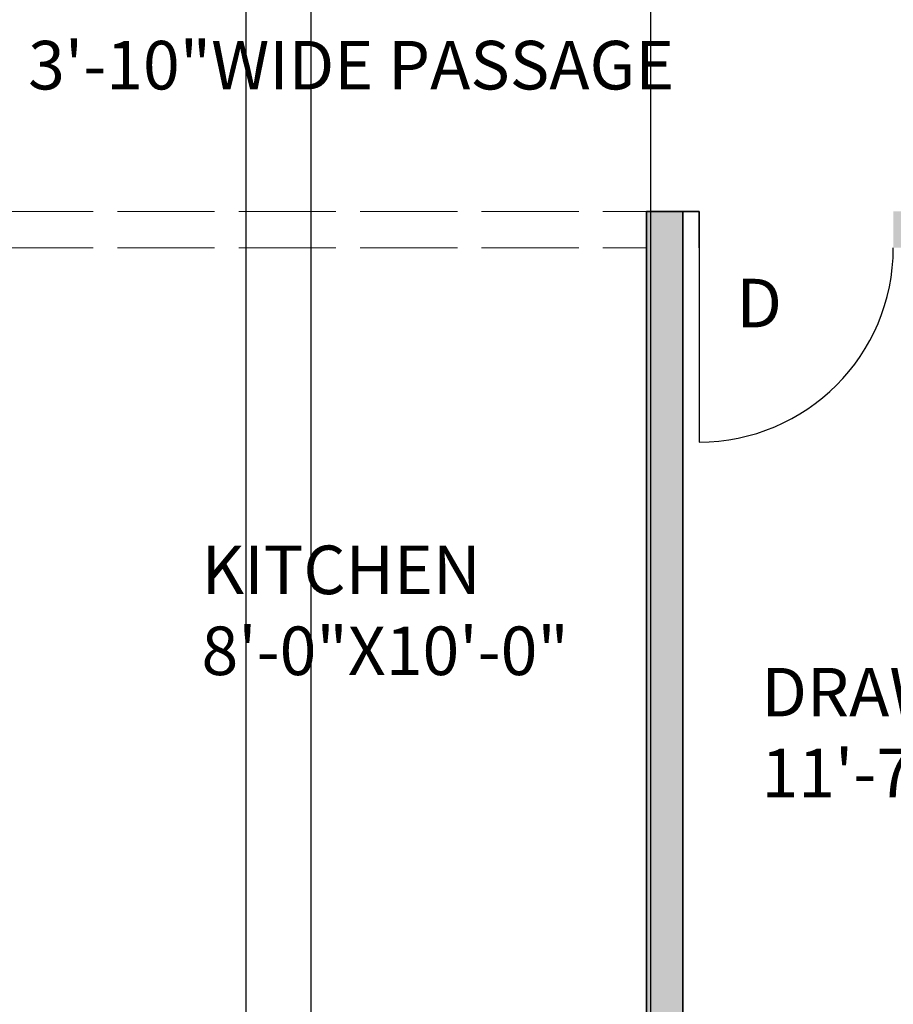
# Model space of a CAD drawing. Units: inches. Extents: x -5 to 330, y -522 to 40.
# Tile 12 of 23: x 51 to 159, y -391 to -269. Entities that reach past the tile are written whole.
import ezdxf

# ---------------------------------------------------------------- set-up
doc = ezdxf.new("R2010")
doc.units = ezdxf.units.IN
doc.header["$MEASUREMENT"] = 0
doc.linetypes.add('ACAD_ISO02W100', pattern=[15, 12, -3])
for name, color, linetype, lineweight in [('A-ANNO-DIMS', 2, 'Continuous', 18), ('A-ANNO-TEXT', 7, 'Continuous', 18), ('A-AREA-IDEN', 7, 'Continuous', 25), ('A-DOOR', 4, 'Continuous', 25), ('A-WALL', 7, 'Continuous', 35), ('A-WALL-OVHD', 8, 'ACAD_ISO02W100', 18)]:
    doc.layers.add(name, color=color, linetype=linetype, lineweight=lineweight)
doc.layers.add('A-WALL-PATT', color=18, linetype='Continuous', lineweight=13, true_color=0x000000)
doc.styles.get("Standard").update_dxf_attribs({"font": 'arial.ttf'})
doc.dimstyles.get("Standard").update_dxf_attribs({"dimtxt": 0.18, "dimasz": 0.18, "dimexe": 0.18, "dimexo": 0.0625, "dimgap": 0.09, "dimtad": 0, "dimtih": 1, "dimtoh": 1, "dimdec": 0, "dimzin": 0, "dimdsep": 46, "dimlunit": 3, "dimtxsty": 'Standard', "dimcen": 0.09, "dimadec": 0, "dimazin": 0, "dimtfac": 1, "dimtdec": 0, "dimtofl": 0, "dimtmove": 0, "dimatfit": 3, "dimfxl": 1, "dimtolj": 1, "dimtzin": 0, "dimarcsym": 0})

# ---------------------------------------------------------------- blocks, each defined once
blk = doc.blocks.new('DOOR-24IN-SWING')
blk.add_line((24, 0), (24, 24))
blk.add_arc((24, 0), 24, 90, 180)
blk = doc.blocks.new('*D40')
at = {"layer": 'A-ANNO-DIMS', "color": 0, "lineweight": -2, "transparency": 16777216}
for p, q in [((32.51, -246.71), (32.51, -522.31)), ((79.01, -246.71), (79.01, -522.31)), ((32.69, -522.13), (55.15, -522.13)), ((78.83, -522.13), (56.37, -522.13))]:
    blk.add_line(p, q, dxfattribs=at)
at = {"layer": 'A-ANNO-DIMS', "color": 0, "transparency": 16777216}
for points in [[(32.69, -522.1), (32.69, -522.16), (32.51, -522.13)], [(78.83, -522.1), (78.83, -522.16), (79.01, -522.13)]]:
    blk.add_solid(points, dxfattribs=at)
at = {"layer": 'Defpoints', "color": 0, "transparency": 16777216}
for p in [(32.51, -246.64), (79.01, -246.64), (79.01, -522.13)]:
    blk.add_point(p, dxfattribs=at)
at = {"layer": 'A-ANNO-DIMS', "color": 0, "transparency": 16777216, "insert": (55.76, -522.13), "char_height": 0.18, "attachment_point": 5}
blk.add_mtext('\\A1;3\'-10 1/2"', dxfattribs=at)
blk = doc.blocks.new('*D41')
at = {"layer": 'A-ANNO-DIMS', "color": 0, "lineweight": -2, "transparency": 16777216}
for p, q in [((87.01, -246.71), (87.01, -522.31)), ((129.01, -246.71), (129.01, -522.31)), ((87.19, -522.13), (107.68, -522.13)), ((128.83, -522.13), (108.34, -522.13))]:
    blk.add_line(p, q, dxfattribs=at)
at = {"layer": 'A-ANNO-DIMS', "color": 0, "transparency": 16777216}
for points in [[(87.19, -522.1), (87.19, -522.16), (87.01, -522.13)], [(128.83, -522.1), (128.83, -522.16), (129.01, -522.13)]]:
    blk.add_solid(points, dxfattribs=at)
at = {"layer": 'Defpoints', "color": 0, "transparency": 16777216}
for p in [(87.01, -246.64), (129.01, -246.64), (129.01, -522.13)]:
    blk.add_point(p, dxfattribs=at)
at = {"layer": 'A-ANNO-DIMS', "color": 0, "transparency": 16777216, "insert": (108.01, -522.13), "char_height": 0.18, "attachment_point": 5}
blk.add_mtext('\\A1;3\'-6"', dxfattribs=at)

msp = doc.modelspace()

# ---------------------------------------------------------------- hatches: boundary and pattern name
at = {"layer": 'A-WALL-PATT'}
h = msp.add_hatch(color=256, dxfattribs=at)
h.dxf.hatch_style = 1
h.paths.add_polyline_path([(164.01, -44.15), (159.51, -44.15), (159.51, -153.14), (164.01, -153.14)], flags=17)
h.paths.add_polyline_path([(224.01, -188.14), (272.01, -188.14), (272.01, -218.14), (260.01, -218.14), (260.01, -222.64), (272.01, -222.64), (272.01, -292.64), (159.01, -292.64), (159.01, -297.14), (272.01, -297.14), (272.01, -417.14), (245.51, -417.14), (245.51, -426.14), (272.01, -426.14), (272.01, -495.14), (281.01, -495.14), (281.01, 12.36), (23.51, 12.36), (23.51, -426.14), (62.92, -426.14), (62.92, -417.14), (32.51, -417.14), (32.51, -297.14), (48.13, -297.14), (48.13, -292.64), (32.51, -292.64), (32.51, -140.64), (133.51, -140.64), (133.51, -131.64), (32.51, -131.64), (32.51, 3.36), (159.51, 3.36), (164.01, 3.36), (220.01, 3.36), (224.51, 3.36), (272.01, 3.36), (272.01, -179.14), (159.51, -179.14), (159.51, -188.14), (219.51, -188.14), (219.51, -266.64), (224.01, -266.64), (224.01, -222.64), (236.01, -222.64), (236.01, -218.14), (224.01, -218.14)])
h.paths.add_polyline_path([(133.01, -292.64), (128.51, -292.64), (128.51, -297.14), (128.51, -417.14), (122.92, -417.14), (122.92, -426.14), (133.01, -426.14)], flags=17)
h.paths.add_polyline_path([(185.51, -417.14), (159.01, -417.14), (159.01, -426.14), (185.51, -426.14)], flags=17)
h.paths.add_polyline_path([(133.51, -140.64), (129.01, -140.64), (129.01, -246.64), (133.51, -246.64)], flags=17)
h.paths.add_polyline_path([(246.01, -48.64), (224.51, -48.64), (224.51, -27.63), (220.01, -27.63), (220.01, -48.64), (198.6, -48.64), (198.6, -53.14), (246.01, -53.14)], flags=17)

# ---------------------------------------------------------------- linework, layer by layer
at = {"layer": 'A-WALL'}
for p, q in [((128.51, -297.14), (128.51, -292.64)), ((128.51, -292.64), (135.01, -292.64)), ((133.01, -292.64), (133.01, -426.14)), ((135.01, -292.64), (135.01, -297.14)), ((128.51, -297.14), (128.51, -417.14))]:
    msp.add_line(p, q, dxfattribs=at)
at = {"layer": 'A-WALL-OVHD'}
for p, q in [((48.13, -292.64), (128.51, -292.64)), ((48.13, -297.14), (128.51, -297.14))]:
    msp.add_line(p, q, dxfattribs=at)

# ---------------------------------------------------------------- block references
at = {"layer": 'A-DOOR', "rotation": 180}
msp.add_blockref('DOOR-24IN-SWING', (159.01, -297.14), dxfattribs=at)

# ---------------------------------------------------------------- texts
at = {"layer": 'A-ANNO-TEXT', "insert": (139.62, -300.97), "char_height": 6, "attachment_point": 1}
msp.add_mtext('D', dxfattribs=at)
at = {"layer": 'A-AREA-IDEN', "char_height": 6, "attachment_point": 1}
for s, insert in [('3\'-10"WIDE PASSAGE', (52.08, -271.57)), ('KITCHEN\\P8\'-0"X10\'-0"', (73.51, -333.93)), ('DRAWING ROOM\\P11\'-7"X10\'-0"', (142.71, -349.04))]:
    msp.add_mtext(s, dxfattribs=dict(at, insert=insert))

# ---------------------------------------------------------------- dimensions: what is measured, and where the dimension line sits
at = {"layer": 'A-ANNO-DIMS'}
for base, p1, p2, picture, middle in [((79.01, -522.13), (32.51, -246.64), (79.01, -246.64), '*D40', (55.76, -522.13)), ((129.01, -522.13), (87.01, -246.64), (129.01, -246.64), '*D41', (108.01, -522.13))]:
    dim = msp.add_linear_dim(base=base, p1=p1, p2=p2, dimstyle='Standard', override={"dimdec": 1, "dimlfac": 1, "dimrnd": 0, "dimzin": 1, "dimdsep": 46, "dimlunit": 4, "dimfrac": 2}, dxfattribs=at)
    dim.commit()
    dim.dimension.update_dxf_attribs({"geometry": picture, "text_midpoint": middle})

doc.saveas('drawing.dxf')
